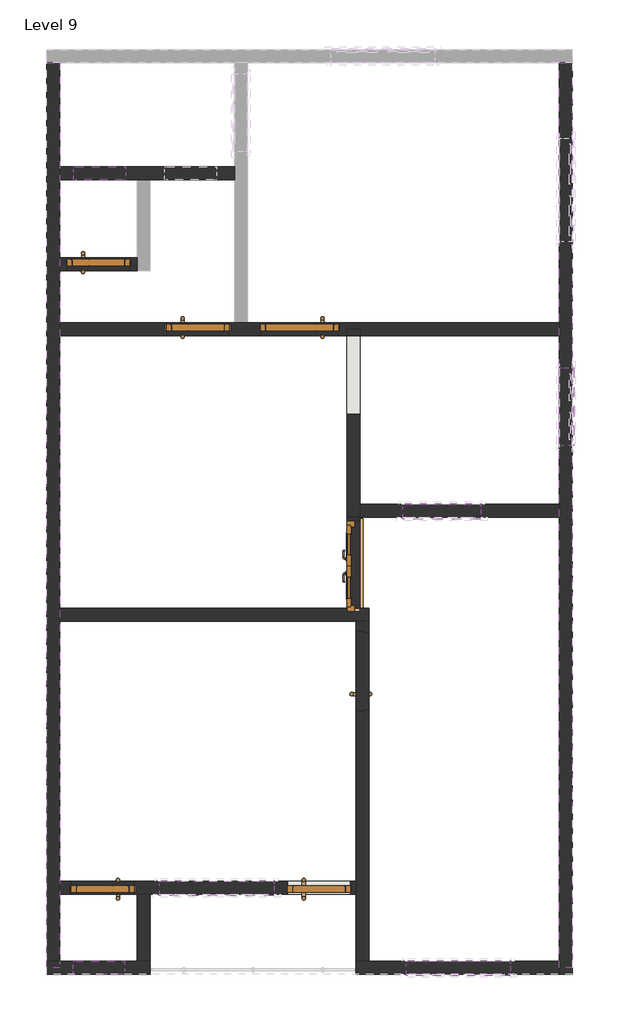
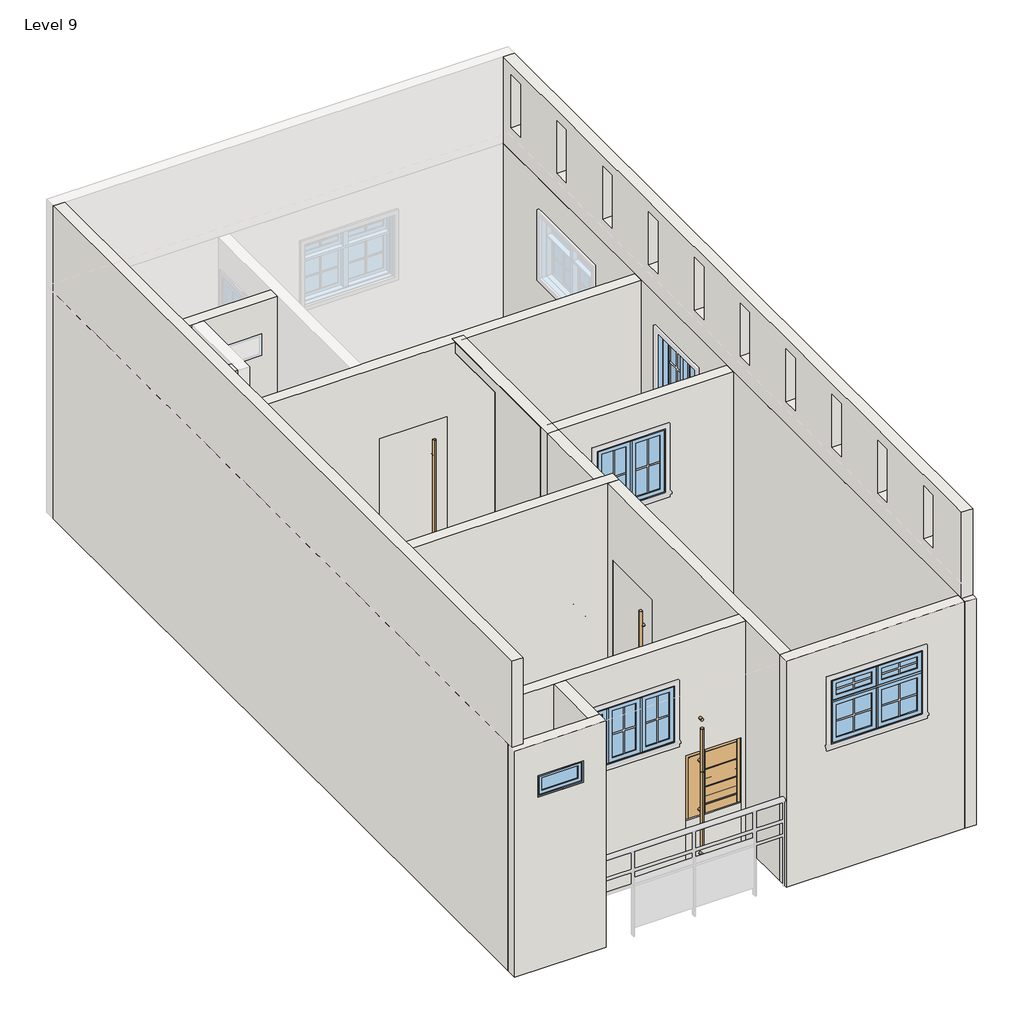
# One storey, part 1 of 2: 25 walls, 8 doors, 8 windows.
"""IFC4 building model written with IfcOpenShell, lengths in millimetres."""

from ifc_helpers import new_model, si_unit, frame, origin, place, context, project, spatial, polyline, outline, extrude, faceted_brep, transform, mapped, element, save
from components import door_9b787682, door_dc81b0c5, door_3_5c4206ef, door_3_79df91aa, door_2576ec39, door_55c03dfd, fixed_2_65c13adb, window_61697a4f, m_window_casement_double_3_e0bd8fa3, m_window_casement_double_awning_double_4_7efa9bbd

model = new_model("IFC4")

# Units and contexts
model_context = context("Model", 3, world=origin())
ifc_project = project(units=[si_unit("LENGTHUNIT", "METRE", prefix="MILLI")], contexts=[model_context])

# Site, building, storey
site = spatial("IfcSite", under=ifc_project)
building = spatial("IfcBuilding", under=site)
storey = spatial("IfcBuildingStorey", under=building, Name="Level 9", Elevation=16611.6)

# Doors
placement = place(None, origin())
door_shape = door_9b787682(model_context)
element("IfcDoor", 1, ObjectType="2'5\"", at=placement, inside=storey, context=model_context, shape_type="MappedRepresentation", body=[
    mapped(door_shape, transform((-22033.2963079, 3049.4742053, 16611.6), x_axis=(1.0, 0.0, 0.0), y_axis=(0.0, 1.0, 0.0), z_axis=(0.0, 0.0, 1.0))),
])
element("IfcDoor", 2, ObjectType="2'5\"", at=placement, inside=storey, context=model_context, shape_type="MappedRepresentation", body=[
    mapped(door_shape, transform((-23201.6963079, 3811.4742053, 16611.6), x_axis=(1.0, 0.0, 0.0), y_axis=(0.0, 1.0, 0.0), z_axis=(0.0, 0.0, 1.0))),
])
element("IfcDoor", 3, ObjectType="2'5\"", at=placement, inside=storey, context=model_context, shape_type="MappedRepresentation", body=[
    mapped(door_shape, transform((-23150.8963079, -3503.7257947, 16611.6), x_axis=(-1.0, 0.0, 0.0), y_axis=(0.0, -1.0, 0.0), z_axis=(0.0, 0.0, 1.0))),
])
door_2_shape = door_dc81b0c5(model_context)
element("IfcDoor", 4, ObjectType="2'5\"", at=placement, inside=storey, context=model_context, shape_type="MappedRepresentation", body=[
    mapped(door_2_shape, transform((-20610.8963079, -3503.7257947, 16657.8445349), x_axis=(1.0, 0.0, 0.0), y_axis=(0.0, 1.0, 0.0), z_axis=(0.0, 0.0, 1.0))),
])
element("IfcDoor", 5, ObjectType="2'5\"", at=placement, inside=storey, context=model_context, shape_type="MappedRepresentation", body=[
    mapped(door_2_shape, transform((-20610.8963079, -3503.7257947, 17267.4445349), x_axis=(1.0, 0.0, 0.0), y_axis=(0.0, 1.0, 0.0), z_axis=(0.0, 0.0, 1.0))),
])
door_3_shape = door_3_5c4206ef(model_context)
element("IfcDoor", 6, ObjectType="3'", at=placement, inside=storey, context=model_context, shape_type="MappedRepresentation", body=[
    mapped(door_3_shape, transform((-20102.8963079, -963.7257947, 16611.6), x_axis=(0.0, 1.0, 0.0), y_axis=(-1.0, 0.0, 0.0), z_axis=(0.0, 0.0, 1.0))),
])
door_3_2_shape = door_3_79df91aa(model_context)
element("IfcDoor", 7, ObjectType="3'", at=placement, inside=storey, context=model_context, shape_type="MappedRepresentation", body=[
    mapped(door_3_2_shape, transform((-20839.4963079, 3049.4742053, 16611.6), x_axis=(-1.0, 0.0, 0.0), y_axis=(0.0, -1.0, 0.0), z_axis=(0.0, 0.0, 1.0))),
])
door_4_shape = door_2576ec39(model_context)
door_5_shape = door_55c03dfd(model_context)
element("IfcDoor", 8, ObjectType="ExtDbl (8) : 3'6\"", at=placement, inside=storey, context=model_context, shape_type="MappedRepresentation", body=[
    mapped(door_4_shape, transform((-20204.4963079, 268.1742053, 16611.6), x_axis=(0.0, -1.0, 0.0), y_axis=(1.0, 0.0, 0.0), z_axis=(0.0, 0.0, 1.0))),
    mapped(door_5_shape, transform((-20204.4963079, 268.1742053, 16611.6), x_axis=(0.0, -1.0, 0.0), y_axis=(1.0, 0.0, 0.0), z_axis=(0.0, 0.0, 1.0))),
])

# Walls
element("IfcWall", 9, ObjectType="Generic - 6\"", at=placement, inside=storey, context=model_context, shape_type="Brep", body=[
    faceted_brep([(-17791.4963079, 6173.6742053, 16611.6), (-17791.4963079, 3125.6742053, 16611.6), (-17791.4963079, 2973.2742053, 16611.6), (-17791.4963079, 992.0742053, 16611.6), (-17791.4963079, 839.6742053, 16611.6), (-17791.4963079, -4367.3257947, 16611.6), (-17791.4963079, -4519.7257947, 16611.6), (-17791.4963079, -4519.7257947, 19812.0), (-17791.4963079, -4367.3257947, 19812.0), (-17791.4963079, 839.6742053, 19812.0), (-17791.4963079, 992.0742053, 19812.0), (-17791.4963079, 2973.2742053, 19812.0), (-17791.4963079, 3125.6742053, 19812.0), (-17791.4963079, 6173.6742053, 19812.0), (-17791.4963079, 4071.8242053, 19340.4), (-17791.4963079, 4071.8242053, 18440.4), (-17791.4963079, 5291.0242053, 18440.4), (-17791.4963079, 5291.0242053, 19340.4), (-17791.4963079, 1682.6367053, 19340.4), (-17791.4963079, 1682.6367053, 18440.4), (-17791.4963079, 2597.0367053, 18440.4), (-17791.4963079, 2597.0367053, 19340.4), (-17639.0963079, 6173.6742053, 16611.6), (-17639.0963079, 6173.6742053, 19812.0), (-17639.0963079, -4519.7257947, 19812.0), (-17639.0963079, -4519.7257947, 16611.6), (-17639.0963079, 4071.8242053, 19340.4), (-17639.0963079, 5291.0242053, 19340.4), (-17639.0963079, 5291.0242053, 18440.4), (-17639.0963079, 4071.8242053, 18440.4), (-17639.0963079, 1682.6367053, 19340.4), (-17639.0963079, 2597.0367053, 19340.4), (-17639.0963079, 2597.0367053, 18440.4), (-17639.0963079, 1682.6367053, 18440.4)], [[[0, 1, 2, 3, 4, 5, 6, 7, 8, 9, 10, 11, 12, 13], [14, 15, 16, 17], [18, 19, 20, 21]], [[22, 23, 24, 25], [26, 27, 28, 29], [30, 31, 32, 33]], [[6, 5, 4, 3, 2, 1, 0, 22, 25]], [[13, 12, 11, 10, 9, 8, 7, 24, 23]], [[0, 13, 23, 22]], [[7, 6, 25, 24]], [[15, 14, 26, 29]], [[16, 15, 29, 28]], [[17, 16, 28, 27]], [[14, 17, 27, 26]], [[19, 18, 30, 33]], [[20, 19, 33, 32]], [[21, 20, 32, 31]], [[18, 21, 31, 30]]]),
])
element("IfcWall", 10, ObjectType="Generic - 6\"", at=placement, inside=storey, context=model_context, shape_type="Brep", body=[
    faceted_brep([(-17791.4963079, -4367.3257947, 16611.6), (-20026.6963079, -4367.3257947, 16611.6), (-20179.0963079, -4367.3257947, 16611.6), (-20179.0963079, -4367.3257947, 19812.0), (-20026.6963079, -4367.3257947, 19812.0), (-17791.4963079, -4367.3257947, 19812.0), (-19585.5697454, -4367.3257947, 19340.4), (-19585.5697454, -4367.3257947, 18440.4), (-18366.3697454, -4367.3257947, 18440.4), (-18366.3697454, -4367.3257947, 19340.4), (-17791.4963079, -4519.7257947, 16611.6), (-17791.4963079, -4519.7257947, 19812.0), (-20179.0963079, -4519.7257947, 19812.0), (-20179.0963079, -4519.7257947, 16611.6), (-19585.5697454, -4519.7257947, 19340.4), (-18366.3697454, -4519.7257947, 19340.4), (-18366.3697454, -4519.7257947, 18440.4), (-19585.5697454, -4519.7257947, 18440.4)], [[[0, 1, 2, 3, 4, 5], [6, 7, 8, 9]], [[10, 11, 12, 13], [14, 15, 16, 17]], [[2, 1, 0, 10, 13]], [[5, 4, 3, 12, 11]], [[0, 5, 11, 10]], [[3, 2, 13, 12]], [[7, 6, 14, 17]], [[8, 7, 17, 16]], [[9, 8, 16, 15]], [[6, 9, 15, 14]]]),
])
element("IfcWall", 11, ObjectType="Generic - 6\"", at=placement, inside=storey, context=model_context, shape_type="Brep", body=[
    faceted_brep([(-23811.2963079, -4519.7257947, 16611.6), (-22592.0963079, -4519.7257947, 16611.6), (-22592.0963079, -4519.7257947, 19812.0), (-23811.2963079, -4519.7257947, 19812.0), (-23500.5431829, -4519.7257947, 19354.8), (-22890.9431829, -4519.7257947, 19354.8), (-22890.9431829, -4519.7257947, 19050.0), (-23500.5431829, -4519.7257947, 19050.0), (-23811.2963079, -4367.3257947, 16611.6), (-23811.2963079, -4367.3257947, 19812.0), (-23658.8963079, -4367.3257947, 19812.0), (-22744.4963079, -4367.3257947, 19812.0), (-22592.0963079, -4367.3257947, 19812.0), (-22592.0963079, -4367.3257947, 16611.6), (-22744.4963079, -4367.3257947, 16611.6), (-23658.8963079, -4367.3257947, 16611.6), (-23500.5431829, -4367.3257947, 19354.8), (-23500.5431829, -4367.3257947, 19050.0), (-22890.9431829, -4367.3257947, 19050.0), (-22890.9431829, -4367.3257947, 19354.8)], [[[0, 1, 2, 3], [4, 5, 6, 7]], [[8, 9, 10, 11, 12, 13, 14, 15], [16, 17, 18, 19]], [[1, 0, 8, 15, 14, 13]], [[3, 2, 12, 11, 10, 9]], [[0, 3, 9, 8]], [[2, 1, 13, 12]], [[17, 16, 4, 7]], [[18, 17, 7, 6]], [[19, 18, 6, 5]], [[16, 19, 5, 4]]]),
])
element("IfcWall", 12, ObjectType="Generic - 6\"", at=placement, inside=storey, context=model_context, shape_type="Brep", body=[
    faceted_brep([(-23658.8963079, -4367.3257947, 16611.6), (-23658.8963079, -3579.9257947, 16611.6), (-23658.8963079, -3427.5257947, 16611.6), (-23658.8963079, -379.5257947, 16611.6), (-23658.8963079, -227.1257947, 16611.6), (-23658.8963079, 2973.2742053, 16611.6), (-23658.8963079, 3125.6742053, 16611.6), (-23658.8963079, 3735.2742053, 16611.6), (-23658.8963079, 3887.6742053, 16611.6), (-23658.8963079, 4802.0742053, 16611.6), (-23658.8963079, 4954.4742053, 16611.6), (-23658.8963079, 6173.6742053, 16611.6), (-23658.8963079, 6173.6742053, 19812.0), (-23658.8963079, 4954.4742053, 19812.0), (-23658.8963079, 4802.0742053, 19812.0), (-23658.8963079, 3887.6742053, 19812.0), (-23658.8963079, 3735.2742053, 19812.0), (-23658.8963079, 3125.6742053, 19812.0), (-23658.8963079, 2973.2742053, 19812.0), (-23658.8963079, -227.1257947, 19812.0), (-23658.8963079, -379.5257947, 19812.0), (-23658.8963079, -3427.5257947, 19812.0), (-23658.8963079, -3579.9257947, 19812.0), (-23658.8963079, -4367.3257947, 19812.0), (-23811.2963079, -4367.3257947, 16611.6), (-23811.2963079, -4367.3257947, 19812.0), (-23811.2963079, 6173.6742053, 19812.0), (-23811.2963079, 6173.6742053, 16611.6)], [[[0, 1, 2, 3, 4, 5, 6, 7, 8, 9, 10, 11, 12, 13, 14, 15, 16, 17, 18, 19, 20, 21, 22, 23]], [[24, 25, 26, 27]], [[11, 10, 9, 8, 7, 6, 5, 4, 3, 2, 1, 0, 24, 27]], [[23, 22, 21, 20, 19, 18, 17, 16, 15, 14, 13, 12, 26, 25]], [[12, 11, 27, 26]], [[0, 23, 25, 24]]]),
])
element("IfcWall", 13, ObjectType="Generic - 6\"", at=placement, inside=storey, context=model_context, shape_type="Brep", body=[
    faceted_brep([(-17791.4963079, 2973.2742053, 19812.0), (-20128.2963079, 2973.2742053, 19812.0), (-20280.6963079, 2973.2742053, 19812.0), (-23658.8963079, 2973.2742053, 19812.0), (-23658.8963079, 2973.2742053, 16611.6), (-22401.5963079, 2973.2742053, 16611.6), (-22401.5963079, 2973.2742053, 18135.6), (-21664.9963079, 2973.2742053, 18135.6), (-21664.9963079, 2973.2742053, 16611.6), (-21296.6963079, 2973.2742053, 16611.6), (-21296.6963079, 2973.2742053, 18801.1), (-20382.2963079, 2973.2742053, 18801.1), (-20382.2963079, 2973.2742053, 16611.6), (-20280.6963079, 2973.2742053, 16611.6), (-20128.2963079, 2973.2742053, 16611.6), (-17791.4963079, 2973.2742053, 16611.6), (-23658.8963079, 3125.6742053, 19812.0), (-21601.4963079, 3125.6742053, 19812.0), (-21449.0963079, 3125.6742053, 19812.0), (-17791.4963079, 3125.6742053, 19812.0), (-17791.4963079, 3125.6742053, 16611.6), (-20382.2963079, 3125.6742053, 16611.6), (-20382.2963079, 3125.6742053, 18801.1), (-21296.6963079, 3125.6742053, 18801.1), (-21296.6963079, 3125.6742053, 16611.6), (-21449.0963079, 3125.6742053, 16611.6), (-21601.4963079, 3125.6742053, 16611.6), (-21664.9963079, 3125.6742053, 16611.6), (-21664.9963079, 3125.6742053, 18135.6), (-22401.5963079, 3125.6742053, 18135.6), (-22401.5963079, 3125.6742053, 16611.6), (-23658.8963079, 3125.6742053, 16611.6), (-22401.5963079, 3105.6742053, 16611.6), (-22416.5963079, 3105.6742053, 16611.6), (-22416.5963079, 3028.6742053, 16611.6), (-22401.5963079, 3028.6742053, 16611.6), (-20382.2963079, 3028.6742053, 16611.6), (-20367.2963079, 3028.6742053, 16611.6), (-20367.2963079, 3105.6742053, 16611.6), (-20382.2963079, 3105.6742053, 16611.6), (-21296.6963079, 3028.6742053, 16611.6), (-21664.9963079, 3028.6742053, 16611.6), (-21649.9963079, 3028.6742053, 16611.6), (-21649.9963079, 3105.6742053, 16611.6), (-21664.9963079, 3105.6742053, 16611.6), (-21296.6963079, 3105.6742053, 16611.6), (-21311.6963079, 3105.6742053, 16611.6), (-21311.6963079, 3028.6742053, 16611.6), (-21296.6963079, 3105.6742053, 18801.1), (-20382.2963079, 3105.6742053, 18801.1), (-20382.2963079, 3028.6742053, 18801.1), (-21296.6963079, 3028.6742053, 18801.1), (-21311.6963079, 3105.6742053, 18816.1), (-20367.2963079, 3105.6742053, 18816.1), (-20367.2963079, 3028.6742053, 18816.1), (-21311.6963079, 3028.6742053, 18816.1), (-21664.9963079, 3105.6742053, 18135.6), (-22401.5963079, 3105.6742053, 18135.6), (-22401.5963079, 3028.6742053, 18135.6), (-21664.9963079, 3028.6742053, 18135.6), (-22416.5963079, 3105.6742053, 18150.6), (-21649.9963079, 3105.6742053, 18150.6), (-21649.9963079, 3028.6742053, 18150.6), (-22416.5963079, 3028.6742053, 18150.6)], [[[0, 1, 2, 3, 4, 5, 6, 7, 8, 9, 10, 11, 12, 13, 14, 15]], [[16, 17, 18, 19, 20, 21, 22, 23, 24, 25, 26, 27, 28, 29, 30, 31]], [[4, 31, 30, 32, 33, 34, 35, 5]], [[20, 15, 14, 13, 12, 36, 37, 38, 39, 21]], [[40, 9, 8, 41, 42, 43, 44, 27, 26, 25, 24, 45, 46, 47]], [[3, 2, 1, 0, 19, 18, 17, 16]], [[0, 15, 20, 19]], [[4, 3, 16, 31]], [[48, 23, 22, 49]], [[50, 11, 10, 51]], [[23, 48, 45, 24]], [[51, 10, 9, 40]], [[49, 22, 21, 39]], [[11, 50, 36, 12]], [[52, 53, 54, 55]], [[52, 55, 47, 46]], [[50, 51, 40, 47, 55, 54, 37, 36]], [[54, 53, 38, 37]], [[48, 49, 39, 38, 53, 52, 46, 45]], [[28, 56, 57, 29]], [[6, 58, 59, 7]], [[56, 28, 27, 44]], [[7, 59, 41, 8]], [[29, 57, 32, 30]], [[58, 6, 5, 35]], [[60, 61, 62, 63]], [[62, 61, 43, 42]], [[59, 58, 35, 34, 63, 62, 42, 41]], [[60, 63, 34, 33]], [[57, 56, 44, 43, 61, 60, 33, 32]]]),
])
element("IfcWall", 14, ObjectType="Generic - 6\"", at=placement, inside=storey, context=model_context, shape_type="Brep", body=[
    faceted_brep([(-20280.6963079, 3049.4742053, 19812.0), (-20280.6963079, 3049.4742053, 16611.6), (-20280.6963079, 839.6742053, 16611.6), (-20280.6963079, 839.6742053, 19812.0), (-20280.6963079, 2974.7724011, 19659.6), (-20280.6963079, 2050.5574639, 19659.6), (-20280.6963079, 2050.5574639, 17221.2), (-20280.6963079, 2974.7724011, 17221.2), (-20128.2963079, 839.6742053, 16611.6), (-20128.2963079, 992.0742053, 16611.6), (-20128.2963079, 3049.4742053, 16611.6), (-20128.2963079, 3049.4742053, 19812.0), (-20128.2963079, 992.0742053, 19812.0), (-20128.2963079, 839.6742053, 19812.0), (-20128.2963079, 2050.5574639, 19659.6), (-20128.2963079, 2974.7724011, 19659.6), (-20128.2963079, 2974.7724011, 17221.2), (-20128.2963079, 2050.5574639, 17221.2)], [[[0, 1, 2, 3], [4, 5, 6, 7]], [[8, 9, 10, 11, 12, 13], [14, 15, 16, 17]], [[2, 1, 10, 9, 8]], [[0, 3, 13, 12, 11]], [[3, 2, 8, 13]], [[4, 15, 14, 5]], [[6, 17, 16, 7]], [[15, 4, 7, 16]], [[5, 14, 17, 6]], [[0, 11, 10, 1]]]),
])
element("IfcWall", 15, ObjectType="Generic - 6\"", at=placement, inside=storey, context=model_context, shape_type="SweptSolid", body=[
    extrude(outline(polyline([(16611.6, -20128.2963079), (16611.6, -17791.4963079), (19812.0, -17791.4963079), (19812.0, -20128.2963079), (16611.6, -20128.2963079)]), holes=[polyline([(19340.4, -19624.1658391), (19340.4, -18709.7658391), (18440.4, -18709.7658391), (18440.4, -19624.1658391), (19340.4, -19624.1658391)])]), frame((0.0, 839.6742053, 0.0), z_axis=(0.0, 1.0, 0.0), x_axis=(0.0, 0.0, 1.0)), (0.0, 0.0, 1.0), 152.4),
])
element("IfcWall", 16, ObjectType="Generic - 6\"", at=placement, inside=storey, context=model_context, shape_type="Brep", body=[
    faceted_brep([(-23658.8963079, -379.5257947, 16611.6), (-20179.0963079, -379.5257947, 16611.6), (-20026.6963079, -379.5257947, 16611.6), (-20026.6963079, -379.5257947, 19812.0), (-20179.0963079, -379.5257947, 19812.0), (-23658.8963079, -379.5257947, 19812.0), (-23658.8963079, -227.1257947, 19812.0), (-20280.6963079, -227.1257947, 19812.0), (-20128.2963079, -227.1257947, 19812.0), (-20026.6963079, -227.1257947, 19812.0), (-20026.6963079, -227.1257947, 16611.6), (-20128.2963079, -227.1257947, 16611.6), (-20128.2963079, -227.1257947, 18721.6), (-20280.6963079, -227.1257947, 18721.6), (-20280.6963079, -227.1257947, 16611.6), (-23658.8963079, -227.1257947, 16611.6), (-20280.6963079, -265.2257947, 16611.6), (-20128.2963079, -265.2257947, 16611.6), (-20280.6963079, -265.2257947, 18721.6), (-20128.2963079, -265.2257947, 18721.6)], [[[0, 1, 2, 3, 4, 5]], [[6, 7, 8, 9, 10, 11, 12, 13, 14, 15]], [[2, 1, 0, 15, 14, 16, 17, 11, 10]], [[5, 4, 3, 9, 8, 7, 6]], [[0, 5, 6, 15]], [[3, 2, 10, 9]], [[18, 16, 14, 13]], [[17, 19, 12, 11]], [[19, 18, 13, 12]], [[16, 18, 19, 17]]]),
])
element("IfcWall", 17, ObjectType="Generic - 6\"", at=placement, inside=storey, context=model_context, shape_type="Brep", body=[
    faceted_brep([(-20179.0963079, -4367.3257947, 19812.0), (-20179.0963079, -3579.9257947, 19812.0), (-20179.0963079, -3427.5257947, 19812.0), (-20179.0963079, -379.5257947, 19812.0), (-20179.0963079, -379.5257947, 16611.6), (-20179.0963079, -506.5257947, 16611.6), (-20179.0963079, -506.5257947, 18801.1), (-20179.0963079, -1420.9257947, 18801.1), (-20179.0963079, -1420.9257947, 16611.6), (-20179.0963079, -3427.5257947, 16611.6), (-20179.0963079, -3579.9257947, 16611.6), (-20179.0963079, -4367.3257947, 16611.6), (-20026.6963079, -379.5257947, 19812.0), (-20026.6963079, -4367.3257947, 19812.0), (-20026.6963079, -4367.3257947, 16611.6), (-20026.6963079, -1420.9257947, 16611.6), (-20026.6963079, -1420.9257947, 18801.1), (-20026.6963079, -506.5257947, 18801.1), (-20026.6963079, -506.5257947, 16611.6), (-20026.6963079, -379.5257947, 16611.6), (-20082.0963079, -506.5257947, 16611.6), (-20082.0963079, -491.5257947, 16611.6), (-20159.0963079, -491.5257947, 16611.6), (-20159.0963079, -506.5257947, 16611.6), (-20159.0963079, -1420.9257947, 16611.6), (-20159.0963079, -1435.9257947, 16611.6), (-20082.0963079, -1435.9257947, 16611.6), (-20082.0963079, -1420.9257947, 16611.6), (-20159.0963079, -506.5257947, 18801.1), (-20159.0963079, -1420.9257947, 18801.1), (-20082.0963079, -1420.9257947, 18801.1), (-20082.0963079, -506.5257947, 18801.1), (-20159.0963079, -1435.9257947, 18816.1), (-20159.0963079, -491.5257947, 18816.1), (-20082.0963079, -491.5257947, 18816.1), (-20082.0963079, -1435.9257947, 18816.1)], [[[0, 1, 2, 3, 4, 5, 6, 7, 8, 9, 10, 11]], [[12, 13, 14, 15, 16, 17, 18, 19]], [[4, 19, 18, 20, 21, 22, 23, 5]], [[14, 11, 10, 9, 8, 24, 25, 26, 27, 15]], [[3, 2, 1, 0, 13, 12]], [[0, 11, 14, 13]], [[4, 3, 12, 19]], [[6, 28, 29, 7]], [[16, 30, 31, 17]], [[28, 6, 5, 23]], [[17, 31, 20, 18]], [[7, 29, 24, 8]], [[30, 16, 15, 27]], [[32, 33, 34, 35]], [[34, 33, 22, 21]], [[31, 30, 27, 26, 35, 34, 21, 20]], [[32, 35, 26, 25]], [[29, 28, 23, 22, 33, 32, 25, 24]]]),
])
element("IfcWall", 18, ObjectType="Generic - 6\"", at=placement, inside=storey, context=model_context, shape_type="Brep", body=[
    faceted_brep([(-20179.0963079, -3579.9257947, 19812.0), (-22592.0963079, -3579.9257947, 19812.0), (-22744.4963079, -3579.9257947, 19812.0), (-23658.8963079, -3579.9257947, 19812.0), (-23658.8963079, -3579.9257947, 16611.6), (-23519.1963079, -3579.9257947, 16611.6), (-23519.1963079, -3579.9257947, 18135.6), (-22782.5963079, -3579.9257947, 18135.6), (-22782.5963079, -3579.9257947, 16611.6), (-22744.4963079, -3579.9257947, 16611.6), (-22592.0963079, -3579.9257947, 16611.6), (-20179.0963079, -3579.9257947, 16611.6), (-22484.1463079, -3579.9257947, 18440.4), (-22484.1463079, -3579.9257947, 19240.4), (-21137.9463079, -3579.9257947, 19240.4), (-21137.9463079, -3579.9257947, 18440.4), (-20979.1963079, -3579.9257947, 18181.8445349), (-20242.5963079, -3579.9257947, 18181.8445349), (-20242.5963079, -3579.9257947, 16657.8445349), (-20979.1963079, -3579.9257947, 16657.8445349), (-23658.8963079, -3427.5257947, 19812.0), (-20179.0963079, -3427.5257947, 19812.0), (-20179.0963079, -3427.5257947, 16611.6), (-22782.5963079, -3427.5257947, 16611.6), (-22782.5963079, -3427.5257947, 18135.6), (-23519.1963079, -3427.5257947, 18135.6), (-23519.1963079, -3427.5257947, 16611.6), (-23658.8963079, -3427.5257947, 16611.6), (-22484.1463079, -3427.5257947, 19240.4), (-22484.1463079, -3427.5257947, 18440.4), (-21137.9463079, -3427.5257947, 18440.4), (-21137.9463079, -3427.5257947, 19240.4), (-20242.5963079, -3427.5257947, 18181.8445349), (-20979.1963079, -3427.5257947, 18181.8445349), (-20979.1963079, -3427.5257947, 16657.8445349), (-20242.5963079, -3427.5257947, 16657.8445349), (-23519.1963079, -3482.9257947, 16611.6), (-23534.1963079, -3482.9257947, 16611.6), (-23534.1963079, -3559.9257947, 16611.6), (-23519.1963079, -3559.9257947, 16611.6), (-22782.5963079, -3559.9257947, 16611.6), (-22767.5963079, -3559.9257947, 16611.6), (-22767.5963079, -3482.9257947, 16611.6), (-22782.5963079, -3482.9257947, 16611.6), (-20979.1963079, -3559.9257947, 18181.8445349), (-20242.5963079, -3559.9257947, 18181.8445349), (-20242.5963079, -3482.9257947, 18181.8445349), (-20979.1963079, -3482.9257947, 18181.8445349), (-20242.5963079, -3559.9257947, 16657.8445349), (-20242.5963079, -3482.9257947, 16657.8445349), (-20227.5963079, -3559.9257947, 16657.8445349), (-20227.5963079, -3482.9257947, 16657.8445349), (-20979.1963079, -3482.9257947, 16657.8445349), (-20994.1963079, -3482.9257947, 16657.8445349), (-20994.1963079, -3559.9257947, 16657.8445349), (-20979.1963079, -3559.9257947, 16657.8445349), (-20994.1963079, -3559.9257947, 18196.8445349), (-20994.1963079, -3482.9257947, 18196.8445349), (-20227.5963079, -3482.9257947, 18196.8445349), (-20227.5963079, -3559.9257947, 18196.8445349), (-23519.1963079, -3559.9257947, 18135.6), (-22782.5963079, -3559.9257947, 18135.6), (-22782.5963079, -3482.9257947, 18135.6), (-23519.1963079, -3482.9257947, 18135.6), (-22767.5963079, -3559.9257947, 18150.6), (-23534.1963079, -3559.9257947, 18150.6), (-23534.1963079, -3482.9257947, 18150.6), (-22767.5963079, -3482.9257947, 18150.6)], [[[0, 1, 2, 3, 4, 5, 6, 7, 8, 9, 10, 11], [12, 13, 14, 15], [16, 17, 18, 19]], [[20, 21, 22, 23, 24, 25, 26, 27], [28, 29, 30, 31], [32, 33, 34, 35]], [[4, 27, 26, 36, 37, 38, 39, 5]], [[22, 11, 10, 9, 8, 40, 41, 42, 43, 23]], [[3, 2, 1, 0, 21, 20]], [[4, 3, 20, 27]], [[0, 11, 22, 21]], [[29, 28, 13, 12]], [[30, 29, 12, 15]], [[31, 30, 15, 14]], [[28, 31, 14, 13]], [[16, 44, 45, 17]], [[32, 46, 47, 33]], [[17, 45, 48, 18]], [[46, 32, 35, 49]], [[18, 48, 50, 51, 49, 35, 34, 52, 53, 54, 55, 19]], [[44, 16, 19, 55]], [[33, 47, 52, 34]], [[56, 57, 58, 59]], [[51, 50, 59, 58]], [[47, 46, 49, 51, 58, 57, 53, 52]], [[54, 53, 57, 56]], [[45, 44, 55, 54, 56, 59, 50, 48]], [[6, 60, 61, 7]], [[24, 62, 63, 25]], [[60, 6, 5, 39]], [[25, 63, 36, 26]], [[7, 61, 40, 8]], [[62, 24, 23, 43]], [[64, 65, 66, 67]], [[66, 65, 38, 37]], [[63, 62, 43, 42, 67, 66, 37, 36]], [[64, 67, 42, 41]], [[61, 60, 39, 38, 65, 64, 41, 40]]]),
])
element("IfcWall", 19, ObjectType="Generic - 6\"", at=placement, inside=storey, context=model_context, shape_type="SweptSolid", body=[
    extrude(outline(polyline([(-22744.4963079, -4367.3257947), (-22744.4963079, -3579.9257947), (-22592.0963079, -3579.9257947), (-22592.0963079, -4367.3257947), (-22744.4963079, -4367.3257947)])), frame((0.0, 0.0, 16611.6), z_axis=(0.0, 0.0, 1.0), x_axis=(1.0, 0.0, 0.0)), (0.0, 0.0, 1.0), 3200.4),
])
element("IfcWall", 20, ObjectType="Generic - 6\"", at=placement, inside=storey, context=model_context, shape_type="Brep", body=[
    faceted_brep([(-23658.8963079, 4802.0742053, 16611.6), (-22744.4963079, 4802.0742053, 16611.6), (-22592.0963079, 4802.0742053, 16611.6), (-21601.4963079, 4802.0742053, 16611.6), (-21601.4963079, 4802.0742053, 19812.0), (-22592.0963079, 4802.0742053, 19812.0), (-22744.4963079, 4802.0742053, 19812.0), (-23658.8963079, 4802.0742053, 19812.0), (-22880.5252141, 4802.0742053, 19354.8), (-22880.5252141, 4802.0742053, 19050.0), (-23490.1252141, 4802.0742053, 19050.0), (-23490.1252141, 4802.0742053, 19354.8), (-21812.6338079, 4802.0742053, 19354.8), (-21812.6338079, 4802.0742053, 19050.0), (-22422.2338079, 4802.0742053, 19050.0), (-22422.2338079, 4802.0742053, 19354.8), (-23658.8963079, 4954.4742053, 16611.6), (-23658.8963079, 4954.4742053, 19812.0), (-21601.4963079, 4954.4742053, 19812.0), (-21601.4963079, 4954.4742053, 16611.6), (-22880.5252141, 4954.4742053, 19354.8), (-23490.1252141, 4954.4742053, 19354.8), (-23490.1252141, 4954.4742053, 19050.0), (-22880.5252141, 4954.4742053, 19050.0), (-21812.6338079, 4954.4742053, 19354.8), (-22422.2338079, 4954.4742053, 19354.8), (-22422.2338079, 4954.4742053, 19050.0), (-21812.6338079, 4954.4742053, 19050.0)], [[[0, 1, 2, 3, 4, 5, 6, 7], [8, 9, 10, 11], [12, 13, 14, 15]], [[16, 17, 18, 19], [20, 21, 22, 23], [24, 25, 26, 27]], [[3, 2, 1, 0, 16, 19]], [[7, 6, 5, 4, 18, 17]], [[0, 7, 17, 16]], [[4, 3, 19, 18]], [[9, 8, 20, 23]], [[10, 9, 23, 22]], [[11, 10, 22, 21]], [[8, 11, 21, 20]], [[13, 12, 24, 27]], [[14, 13, 27, 26]], [[15, 14, 26, 25]], [[12, 15, 25, 24]]]),
])
element("IfcWall", 21, ObjectType="Generic - 6\"", at=placement, inside=storey, context=model_context, shape_type="Brep", body=[
    faceted_brep([(-22744.4963079, 3735.2742053, 19812.0), (-23658.8963079, 3735.2742053, 19812.0), (-23658.8963079, 3735.2742053, 16611.6), (-23569.9963079, 3735.2742053, 16611.6), (-23569.9963079, 3735.2742053, 18135.6), (-22833.3963079, 3735.2742053, 18135.6), (-22833.3963079, 3735.2742053, 16611.6), (-22744.4963079, 3735.2742053, 16611.6), (-23658.8963079, 3887.6742053, 19812.0), (-22744.4963079, 3887.6742053, 19812.0), (-22744.4963079, 3887.6742053, 16611.6), (-22833.3963079, 3887.6742053, 16611.6), (-22833.3963079, 3887.6742053, 18135.6), (-23569.9963079, 3887.6742053, 18135.6), (-23569.9963079, 3887.6742053, 16611.6), (-23658.8963079, 3887.6742053, 16611.6), (-23569.9963079, 3867.6742053, 16611.6), (-23584.9963079, 3867.6742053, 16611.6), (-23584.9963079, 3790.6742053, 16611.6), (-23569.9963079, 3790.6742053, 16611.6), (-22833.3963079, 3790.6742053, 16611.6), (-22818.3963079, 3790.6742053, 16611.6), (-22818.3963079, 3867.6742053, 16611.6), (-22833.3963079, 3867.6742053, 16611.6), (-22833.3963079, 3867.6742053, 18135.6), (-23569.9963079, 3867.6742053, 18135.6), (-23569.9963079, 3790.6742053, 18135.6), (-22833.3963079, 3790.6742053, 18135.6), (-23584.9963079, 3867.6742053, 18150.6), (-22818.3963079, 3867.6742053, 18150.6), (-22818.3963079, 3790.6742053, 18150.6), (-23584.9963079, 3790.6742053, 18150.6)], [[[0, 1, 2, 3, 4, 5, 6, 7]], [[8, 9, 10, 11, 12, 13, 14, 15]], [[2, 15, 14, 16, 17, 18, 19, 3]], [[10, 7, 6, 20, 21, 22, 23, 11]], [[1, 0, 9, 8]], [[0, 7, 10, 9]], [[2, 1, 8, 15]], [[12, 24, 25, 13]], [[4, 26, 27, 5]], [[24, 12, 11, 23]], [[5, 27, 20, 6]], [[13, 25, 16, 14]], [[26, 4, 3, 19]], [[28, 29, 30, 31]], [[30, 29, 22, 21]], [[27, 26, 19, 18, 31, 30, 21, 20]], [[28, 31, 18, 17]], [[25, 24, 23, 22, 29, 28, 17, 16]]]),
])
element("IfcWall", 22, ObjectType="Generic - 6\"", at=placement, inside=storey, context=model_context, shape_type="Brep", body=[
    faceted_brep([(-20280.6963079, -227.1257947, 19812.0), (-20280.6963079, 839.6742053, 19812.0), (-20280.6963079, 839.6742053, 16611.6), (-20280.6963079, 801.5742053, 16611.6), (-20280.6963079, 801.5742053, 18721.6), (-20280.6963079, -227.1257947, 18721.6), (-20128.2963079, 839.6742053, 19812.0), (-20128.2963079, -227.1257947, 19812.0), (-20128.2963079, -227.1257947, 18721.6), (-20128.2963079, 801.5742053, 18721.6), (-20128.2963079, 801.5742053, 16611.6), (-20128.2963079, 839.6742053, 16611.6), (-20179.0963079, -227.1257947, 19812.0), (-20179.0963079, -227.1257947, 18721.6)], [[[0, 1, 2, 3, 4, 5]], [[6, 7, 8, 9, 10, 11]], [[2, 11, 10, 3]], [[1, 0, 12, 7, 6]], [[2, 1, 6, 11]], [[7, 12, 0, 5, 13, 8]], [[4, 9, 8, 13, 5]], [[9, 4, 3, 10]]]),
])
element("IfcWall", 23, ObjectType="Generic - 6\"", at=placement, inside=storey, context=model_context, shape_type="Brep", body=[
    faceted_brep([(-23658.8963079, 2973.2742053, 16611.6), (-20280.6963079, 2973.2742053, 16611.6), (-20128.2963079, 2973.2742053, 16611.6), (-17791.4963079, 2973.2742053, 16611.6), (-17791.4963079, 2973.2742053, 19812.0), (-20128.2963079, 2973.2742053, 19812.0), (-20280.6963079, 2973.2742053, 19812.0), (-23658.8963079, 2973.2742053, 19812.0), (-23658.8963079, 3125.6742053, 16611.6), (-23658.8963079, 3125.6742053, 19812.0), (-21601.4963079, 3125.6742053, 19812.0), (-21449.0963079, 3125.6742053, 19812.0), (-17791.4963079, 3125.6742053, 19812.0), (-17791.4963079, 3125.6742053, 16611.6), (-21449.0963079, 3125.6742053, 16611.6), (-21601.4963079, 3125.6742053, 16611.6)], [[[0, 1, 2, 3, 4, 5, 6, 7]], [[8, 9, 10, 11, 12, 13, 14, 15]], [[3, 2, 1, 0, 8, 15, 14, 13]], [[7, 6, 5, 4, 12, 11, 10, 9]], [[0, 7, 9, 8]], [[4, 3, 13, 12]]]),
])
element("IfcWall", 24, ObjectType="Generic - 6\"", at=placement, inside=storey, context=model_context, shape_type="SweptSolid", body=[
    extrude(outline(polyline([(2973.2742053, 16611.6), (992.0742053, 16611.6), (992.0742053, 19812.0), (2973.2742053, 19812.0), (2973.2742053, 19659.6), (2050.5574639, 19659.6), (2050.5574639, 17221.2), (2973.2742053, 17221.2), (2973.2742053, 16611.6)])), frame((-20280.6963079, 0.0, 0.0), z_axis=(1.0, 0.0, 0.0), x_axis=(0.0, 1.0, 0.0)), (0.0, 0.0, 1.0), 152.4),
])
element("IfcWall", 25, ObjectType="Generic - 6\"", at=placement, inside=storey, context=model_context, shape_type="SweptSolid", body=[
    extrude(outline(polyline([(16611.6, -20128.2963079), (16611.6, -17791.4963079), (19812.0, -17791.4963079), (19812.0, -20128.2963079), (16611.6, -20128.2963079)]), holes=[polyline([(19340.4, -19624.1658391), (19340.4, -18709.7658391), (18440.4, -18709.7658391), (18440.4, -19624.1658391), (19340.4, -19624.1658391)])]), frame((0.0, 839.6742053, 0.0), z_axis=(0.0, 1.0, 0.0), x_axis=(0.0, 0.0, 1.0)), (0.0, 0.0, 1.0), 152.4),
])
element("IfcWall", 26, ObjectType="Generic - 6\"", at=placement, inside=storey, context=model_context, shape_type="Brep", body=[
    faceted_brep([(-23658.8963079, -379.5257947, 16611.6), (-20179.0963079, -379.5257947, 16611.6), (-20179.0963079, -379.5257947, 19812.0), (-23658.8963079, -379.5257947, 19812.0), (-23658.8963079, -227.1257947, 19812.0), (-20280.6963079, -227.1257947, 19812.0), (-20179.0963079, -227.1257947, 19812.0), (-20179.0963079, -227.1257947, 18721.6), (-20280.6963079, -227.1257947, 18721.6), (-20280.6963079, -227.1257947, 16611.6), (-23658.8963079, -227.1257947, 16611.6), (-20280.6963079, -265.2257947, 16611.6), (-20179.0963079, -265.2257947, 16611.6), (-20179.0963079, -265.2257947, 18721.6), (-20280.6963079, -265.2257947, 18721.6)], [[[0, 1, 2, 3]], [[4, 5, 6, 7, 8, 9, 10]], [[1, 0, 10, 9, 11, 12]], [[3, 2, 6, 5, 4]], [[2, 1, 12, 13, 7, 6]], [[14, 11, 9, 8]], [[11, 14, 13, 12]], [[14, 8, 7, 13]], [[0, 3, 4, 10]]]),
])
element("IfcWall", 27, ObjectType="Generic - 6\"", at=placement, inside=storey, context=model_context, shape_type="Brep", body=[
    faceted_brep([(-20179.0963079, -379.5257947, 16611.6), (-20179.0963079, -3427.5257947, 16611.6), (-20179.0963079, -3579.9257947, 16611.6), (-20179.0963079, -4367.3257947, 16611.6), (-20179.0963079, -4367.3257947, 19812.0), (-20179.0963079, -3579.9257947, 19812.0), (-20179.0963079, -3427.5257947, 19812.0), (-20179.0963079, -379.5257947, 19812.0), (-20026.6963079, -379.5257947, 16611.6), (-20026.6963079, -379.5257947, 19812.0), (-20026.6963079, -4367.3257947, 19812.0), (-20026.6963079, -4367.3257947, 16611.6)], [[[0, 1, 2, 3, 4, 5, 6, 7]], [[8, 9, 10, 11]], [[3, 2, 1, 0, 8, 11]], [[7, 6, 5, 4, 10, 9]], [[4, 3, 11, 10]], [[0, 7, 9, 8]]]),
])
element("IfcWall", 28, ObjectType="Generic - 6\"", at=placement, inside=storey, context=model_context, shape_type="Brep", body=[
    faceted_brep([(-23658.8963079, -3579.9257947, 16611.6), (-22744.4963079, -3579.9257947, 16611.6), (-22592.0963079, -3579.9257947, 16611.6), (-20179.0963079, -3579.9257947, 16611.6), (-20179.0963079, -3579.9257947, 19812.0), (-22592.0963079, -3579.9257947, 19812.0), (-22744.4963079, -3579.9257947, 19812.0), (-23658.8963079, -3579.9257947, 19812.0), (-22484.1463079, -3579.9257947, 18440.4), (-22484.1463079, -3579.9257947, 19240.4), (-21137.9463079, -3579.9257947, 19240.4), (-21137.9463079, -3579.9257947, 18440.4), (-20979.1963079, -3579.9257947, 18791.4445349), (-20242.5963079, -3579.9257947, 18791.4445349), (-20242.5963079, -3579.9257947, 17267.4445349), (-20979.1963079, -3579.9257947, 17267.4445349), (-20179.0963079, -3427.5257947, 16611.6), (-23658.8963079, -3427.5257947, 16611.6), (-23658.8963079, -3427.5257947, 19812.0), (-20179.0963079, -3427.5257947, 19812.0), (-22484.1463079, -3427.5257947, 19240.4), (-22484.1463079, -3427.5257947, 18440.4), (-21137.9463079, -3427.5257947, 18440.4), (-21137.9463079, -3427.5257947, 19240.4), (-20242.5963079, -3427.5257947, 18791.4445349), (-20979.1963079, -3427.5257947, 18791.4445349), (-20979.1963079, -3427.5257947, 17267.4445349), (-20242.5963079, -3427.5257947, 17267.4445349), (-20979.1963079, -3559.9257947, 18791.4445349), (-20242.5963079, -3559.9257947, 18791.4445349), (-20242.5963079, -3482.9257947, 18791.4445349), (-20979.1963079, -3482.9257947, 18791.4445349), (-20242.5963079, -3559.9257947, 17267.4445349), (-20242.5963079, -3482.9257947, 17267.4445349), (-20227.5963079, -3559.9257947, 17267.4445349), (-20227.5963079, -3482.9257947, 17267.4445349), (-20979.1963079, -3482.9257947, 17267.4445349), (-20994.1963079, -3482.9257947, 17267.4445349), (-20994.1963079, -3559.9257947, 17267.4445349), (-20979.1963079, -3559.9257947, 17267.4445349), (-20994.1963079, -3559.9257947, 18806.4445349), (-20994.1963079, -3482.9257947, 18806.4445349), (-20227.5963079, -3482.9257947, 18806.4445349), (-20227.5963079, -3559.9257947, 18806.4445349)], [[[0, 1, 2, 3, 4, 5, 6, 7], [8, 9, 10, 11], [12, 13, 14, 15]], [[16, 17, 18, 19], [20, 21, 22, 23], [24, 25, 26, 27]], [[3, 2, 1, 0, 17, 16]], [[7, 6, 5, 4, 19, 18]], [[4, 3, 16, 19]], [[21, 20, 9, 8]], [[22, 21, 8, 11]], [[23, 22, 11, 10]], [[20, 23, 10, 9]], [[12, 28, 29, 13]], [[24, 30, 31, 25]], [[13, 29, 32, 14]], [[30, 24, 27, 33]], [[14, 32, 34, 35, 33, 27, 26, 36, 37, 38, 39, 15]], [[28, 12, 15, 39]], [[25, 31, 36, 26]], [[40, 41, 42, 43]], [[35, 34, 43, 42]], [[31, 30, 33, 35, 42, 41, 37, 36]], [[38, 37, 41, 40]], [[29, 28, 39, 38, 40, 43, 34, 32]], [[0, 7, 18, 17]]]),
])
element("IfcWall", 29, ObjectType="Generic - 6\"", at=placement, inside=storey, context=model_context, shape_type="SweptSolid", body=[
    extrude(outline(polyline([(-22744.4963079, -4367.3257947), (-22744.4963079, -3579.9257947), (-22592.0963079, -3579.9257947), (-22592.0963079, -4367.3257947), (-22744.4963079, -4367.3257947)])), frame((0.0, 0.0, 16611.6), z_axis=(0.0, 0.0, 1.0), x_axis=(1.0, 0.0, 0.0)), (0.0, 0.0, 1.0), 3200.4),
])
element("IfcWall", 30, ObjectType="Generic - 6\"", at=placement, inside=storey, context=model_context, shape_type="SweptSolid", body=[
    extrude(outline(polyline([(-22744.4963079, 3735.2742053), (-23658.8963079, 3735.2742053), (-23658.8963079, 3887.6742053), (-22744.4963079, 3887.6742053), (-22744.4963079, 3735.2742053)])), frame((0.0, 0.0, 16611.6), z_axis=(0.0, 0.0, 1.0), x_axis=(1.0, 0.0, 0.0)), (0.0, 0.0, 1.0), 3200.4),
])
element("IfcWall", 31, ObjectType="Generic - 6\"", at=placement, inside=storey, context=model_context, shape_type="Brep", body=[
    faceted_brep([(-20280.6963079, 839.6742053, 16611.6), (-20280.6963079, -227.1257947, 16611.6), (-20280.6963079, -227.1257947, 19812.0), (-20280.6963079, 839.6742053, 19812.0), (-20128.2963079, 839.6742053, 16611.6), (-20128.2963079, 839.6742053, 19812.0), (-20128.2963079, -227.1257947, 19812.0), (-20128.2963079, -227.1257947, 16611.6), (-20179.0963079, -227.1257947, 19812.0)], [[[0, 1, 2, 3]], [[4, 5, 6, 7]], [[1, 0, 4, 7]], [[3, 2, 8, 6, 5]], [[2, 1, 7, 6, 8]], [[0, 3, 5, 4]]]),
])
element("IfcWall", 32, ObjectType="Generic - 6\"", at=placement, inside=storey, context=model_context, shape_type="SweptSolid", body=[
    extrude(outline(polyline([(6173.6742053, 19812.0), (-4443.5257947, 19812.0), (-4443.5257947, 21031.2), (6173.6742053, 21031.2), (6173.6742053, 19812.0)]), holes=[polyline([(-3566.483991, 20875.4336528), (-3781.9528499, 20875.4336528), (-3781.9528499, 20127.6299662), (-3566.483991, 20127.6299662), (-3566.483991, 20875.4336528)]), polyline([(5774.7247726, 20140.2538824), (5990.1936315, 20140.2538824), (5990.1936315, 20888.0575691), (5774.7247726, 20888.0575691), (5774.7247726, 20140.2538824)]), polyline([(4928.3405623, 20138.8512251), (4928.3405623, 20886.6549117), (4712.8717035, 20886.6549117), (4712.8717035, 20138.8512251), (4928.3405623, 20138.8512251)]), polyline([(3866.4874932, 20137.4485677), (3866.4874932, 20885.2522543), (3651.0186343, 20885.2522543), (3651.0186343, 20137.4485677), (3866.4874932, 20137.4485677)]), polyline([(2804.634424, 20136.0459103), (2804.634424, 20883.849597), (2589.1655651, 20883.849597), (2589.1655651, 20136.0459103), (2804.634424, 20136.0459103)]), polyline([(1742.7813548, 20134.643253), (1742.7813548, 20882.4469396), (1527.312496, 20882.4469396), (1527.312496, 20134.643253), (1742.7813548, 20134.643253)]), polyline([(680.9282857, 20133.2405956), (680.9282857, 20881.0442823), (465.4594268, 20881.0442823), (465.4594268, 20133.2405956), (680.9282857, 20133.2405956)]), polyline([(-380.9247835, 20131.8379382), (-380.9247835, 20879.6416249), (-596.3936424, 20879.6416249), (-596.3936424, 20131.8379382), (-380.9247835, 20131.8379382)]), polyline([(-1442.7778527, 20130.4352809), (-1442.7778527, 20878.2389675), (-1658.2467115, 20878.2389675), (-1658.2467115, 20130.4352809), (-1442.7778527, 20130.4352809)]), polyline([(-2504.6309218, 20876.8363102), (-2720.0997807, 20876.8363102), (-2720.0997807, 20129.0326235), (-2504.6309218, 20129.0326235), (-2504.6309218, 20876.8363102)])]), frame((-17791.4963079, 0.0, 0.0), z_axis=(1.0, 0.0, 0.0), x_axis=(0.0, 1.0, 0.0)), (0.0, 0.0, 1.0), 152.4),
])
element("IfcWall", 33, ObjectType="Generic - 6\"", at=placement, inside=storey, context=model_context, shape_type="Brep", body=[
    faceted_brep([(-23811.2963079, 6173.6742053, 19812.0), (-23811.2963079, -4443.5257947, 19812.0), (-23811.2963079, -4443.5257947, 21031.2), (-23811.2963079, 6173.6742053, 21031.2), (-23658.8963079, 6173.6742053, 19812.0), (-23658.8963079, 6173.6742053, 21031.2), (-23658.8963079, -4443.5257947, 21031.2), (-23658.8963079, -4443.5257947, 19812.0), (-23658.8963079, -4367.3257947, 19812.0)], [[[0, 1, 2, 3]], [[4, 5, 6, 7, 8]], [[1, 0, 4, 8, 7]], [[2, 1, 7, 6]], [[3, 2, 6, 5]], [[0, 3, 5, 4]]]),
])

# Windows
fixed_2_shape = fixed_2_65c13adb(model_context)
element("IfcWindow", 34, ObjectType="Fixed : 2'", at=placement, inside=storey, context=model_context, shape_type="MappedRepresentation", body=[
    mapped(fixed_2_shape, transform((-23233.8431829, -4443.5257947, 18135.6), x_axis=(-1.0, 0.0, 0.0), y_axis=(0.0, -1.0, 0.0), z_axis=(0.0, 0.0, 1.0))),
])
element("IfcWindow", 35, ObjectType="Fixed : 2'", at=placement, inside=storey, context=model_context, shape_type="MappedRepresentation", body=[
    mapped(fixed_2_shape, transform((-23147.2252141, 4878.2742053, 18135.6), x_axis=(1.0, 0.0, 0.0), y_axis=(0.0, 1.0, 0.0), z_axis=(0.0, 0.0, 1.0))),
])
window_shape = window_61697a4f(model_context)
element("IfcWindow", 36, ObjectType="M_Window-Awning-Triple-Horizontal : 4'5\"", at=placement, inside=storey, context=model_context, shape_type="MappedRepresentation", body=[
    mapped(window_shape, transform((-21811.0463079, -3503.7257947, 17540.4), x_axis=(-1.0, 0.0, 0.0), y_axis=(0.0, -1.0, 0.0), z_axis=(0.0, 0.0, 1.0))),
])
element("IfcWindow", 37, ObjectType="M_Window-Awning-Triple-Horizontal : 4'5\"", at=placement, inside=storey, context=model_context, shape_type="MappedRepresentation", body=[
    mapped(window_shape, transform((-21811.0463079, -3503.7257947, 17540.4), x_axis=(-1.0, 0.0, 0.0), y_axis=(0.0, -1.0, 0.0), z_axis=(0.0, 0.0, 1.0))),
])
m_window_casement_double_3_shape = m_window_casement_double_3_e0bd8fa3(model_context)
element("IfcWindow", 38, ObjectType="M_Window-Casement-Double : 3'", at=placement, inside=storey, context=model_context, shape_type="MappedRepresentation", body=[
    mapped(m_window_casement_double_3_shape, transform((-19166.9658391, 915.8742053, 17540.4), x_axis=(-1.0, 0.0, 0.0), y_axis=(0.0, -1.0, 0.0), z_axis=(0.0, 0.0, 1.0))),
])
element("IfcWindow", 39, ObjectType="M_Window-Casement-Double : 3'", at=placement, inside=storey, context=model_context, shape_type="MappedRepresentation", body=[
    mapped(m_window_casement_double_3_shape, transform((-17715.2963079, 2139.8367053, 17540.4), x_axis=(0.0, -1.0, 0.0), y_axis=(1.0, 0.0, 0.0), z_axis=(0.0, 0.0, 1.0))),
])
element("IfcWindow", 40, ObjectType="M_Window-Casement-Double : 3'", at=placement, inside=storey, context=model_context, shape_type="MappedRepresentation", body=[
    mapped(m_window_casement_double_3_shape, transform((-19166.9658391, 915.8742053, 17540.4), x_axis=(-1.0, 0.0, 0.0), y_axis=(0.0, -1.0, 0.0), z_axis=(0.0, 0.0, 1.0))),
])
m_window_casement_double_awning_double_4_shape = m_window_casement_double_awning_double_4_7efa9bbd(model_context)
element("IfcWindow", 41, ObjectType="M_Window-Casement-Double-Awning-Double : 4'", at=placement, inside=storey, context=model_context, shape_type="MappedRepresentation", body=[
    mapped(m_window_casement_double_awning_double_4_shape, transform((-18975.9697454, -4443.5257947, 17540.4), x_axis=(-1.0, 0.0, 0.0), y_axis=(0.0, -1.0, 0.0), z_axis=(0.0, 0.0, 1.0))),
])

save(model, "model.ifc")

# Revit data of these elements
# Type "2'5\""
#   Type Mark = "9"
#   Water resistance = "up to Class E900, EN 12208:2001"
#   Uniclass2015Version = "v1.21"
#   Uniclass2015Reference = "Ss_25_30_20_30"
#   Uniclass2015Description = "Frame and door leaf system"
#   URL = "www.aluprof.com"
#   Type IFC Predefined Type = "USERDEFINED"
#   Right-hand / Left-hand door [instance default] = ""
#   Resistance to wind load = "up to Class C5/B5, EN 12210:2001"
#   Insert type = "ST"
#   Hardware [instance default] = ""
#   Product page = "https://aluprof.com/en/architects/offer/window-and-door-systems/panel-doors#visualisation"
#   Operation = "SinglePanelOutwardOpening"
#   Opening type = "Outward"
#   NBSReference = "25-50-20/125"
#   NBSDescription = "Frame and door leaf system"
#   Important = "The actual acceptable construction dimensions are dependent on the selection of profiles and hardware, glazing type, construction weight and the construction’s operating conditions. These should be determined by a suitably qualified person, and using ALUPROF’s calculation software"
#   IfcExportType = "USERDEFINED"
#   IfcExportAs = "IfcDoorType"
#   Handle type [instance default] = ""
#   Manufacturer = "ALUPROF SA"
#   Export Type to IFC As = "IfcDoorType"
#   Door sill type [instance default] = ""
#   Description = "External single-leaf panel door outward opening"
#   Model = "MB-86 ST Panel Door AD07"
#   Content of the recyclate in the material = "69.2%"
#   COBie.Type.WarrantyDurationParts = ""
#   COBie.Type.Name = ""
#   COBie.Type.Manufacturer = "ALUPROF SA"
#   COBie.Space.Name = ""
#   COBie.Floor.Name = ""
#   COBie.Facility.Name = ""
#   COBie.CreatedOn = ""
#   COBie.Component.WarrantyStartDate = ""
#   COBie.Component.Name = "MB-86 ST Panel Door AD07"
#   Burglar resistance = "RC2"
#   Air permeability = "up to Class 4, EN 12207:2001"
#   Width of the active leaf = 2' - 1.17717"
#   Placement in wall = 0' - 0.7874"
#   Thickness = 0' - 3.0315"
#   Height of the opening sash = 4' - 9.44094"
#   Handle Offset = 3' - 5.33858"
#   Rough Height = 5' - 2.40945"
#   Rough Width = 2' - 6.1811"
#   Height = 5' - 0"
#   Width = 2' - 5"
#   Construction depth = 0' - 3.0315"
#   Clear opening width = 1' - 8.94882"
#   Clear opening height = 4' - 8.47638"
#   Height of the array = 0' - 9.08136"
#   Schedule No. [instance default] = 1
#   Handrail [instance default] = yes
#   IsExternal = yes
#   Handle [instance default] = no
#   Door closer [instance default] = no
#   Function = 1
#   COBie.Type = yes
#   COBie = yes
#   Access control [instance default] = no
#   Panel = element 346771
#   Wall Closure = (empty or 0)
# Type "3'"
#   Type Mark = "10"
#   Water resistance = "up to Class E900, EN 12208:2001"
#   Uniclass2015Version = "v1.21"
#   Uniclass2015Reference = "Ss_25_30_20_30"
#   Uniclass2015Description = "Frame and door leaf system"
#   URL = "www.aluprof.com"
#   Type IFC Predefined Type = "USERDEFINED"
#   Right-hand / Left-hand door [instance default] = ""
#   Resistance to wind load = "up to Class C5/B5, EN 12210:2001"
#   Insert type = "ST"
#   Hardware [instance default] = ""
#   Product page = "https://aluprof.com/en/architects/offer/window-and-door-systems/panel-doors#visualisation"
#   Operation = "SinglePanelOutwardOpening"
#   Opening type = "Outward"
#   NBSReference = "25-50-20/125"
#   NBSDescription = "Frame and door leaf system"
#   Important = "The actual acceptable construction dimensions are dependent on the selection of profiles and hardware, glazing type, construction weight and the construction’s operating conditions. These should be determined by a suitably qualified person, and using ALUPROF’s calculation software"
#   IfcExportType = "USERDEFINED"
#   IfcExportAs = "IfcDoorType"
#   Handle type [instance default] = ""
#   Manufacturer = "ALUPROF SA"
#   Export Type to IFC As = "IfcDoorType"
#   Door sill type [instance default] = ""
#   Description = "External single-leaf panel door outward opening"
#   Model = "MB-86 ST Panel Door AD07"
#   Content of the recyclate in the material = "69.2%"
#   COBie.Type.WarrantyDurationParts = ""
#   COBie.Type.Name = ""
#   COBie.Type.Manufacturer = "ALUPROF SA"
#   COBie.Space.Name = ""
#   COBie.Floor.Name = ""
#   COBie.Facility.Name = ""
#   COBie.CreatedOn = ""
#   COBie.Component.WarrantyStartDate = ""
#   COBie.Component.Name = "MB-86 ST Panel Door AD07"
#   Burglar resistance = "RC2"
#   Air permeability = "up to Class 4, EN 12207:2001"
#   Width of the active leaf = 2' - 8.17717"
#   Placement in wall = 0' - 0.7874"
#   Thickness = 0' - 3.0315"
#   Height of the opening sash = 6' - 11.64173"
#   Handle Offset = 3' - 5.33858"
#   Rough Height = 7' - 4.61024"
#   Rough Width = 3' - 1.1811"
#   Height = 7' - 2.20079"
#   Width = 3' - 0"
#   Construction depth = 0' - 3.0315"
#   Clear opening width = 2' - 3.94882"
#   Clear opening height = 6' - 10.67717"
#   Height of the array = 1' - 1.44816"
#   Schedule No. [instance default] = 1
#   Handrail [instance default] = yes
#   IsExternal = yes
#   Handle [instance default] = no
#   Door closer [instance default] = no
#   Function = 1
#   COBie.Type = yes
#   COBie = yes
#   Access control [instance default] = no
#   Panel = element 346771
#   Wall Closure = (empty or 0)
# Type "ExtDbl (8) : 3'6\""
#   Type Mark = "14"
#   Operation = "DoubleDoorSingleSwing"
#   Keynote = "L20"
#   Wrap Layers (Int) from Ext = 0' - 6.98819"
#   Wrap Layers (Ext) from Ext = 0' - 4.03543"
#   Top of Lock Rail = 2' - 11.43307"
#   Thickness = 0' - 1.73228"
#   Stile Shutting = 0' - 4.92126"
#   Stile - Top Rail = 0' - 5.90551"
#   Stile - Lock Rail = 0' - 5.90551"
#   Stile - Hanging = 0' - 3.93701"
#   Stile - Bottom Rail = 0' - 11.81102"
#   Rough Width = 3' - 6"
#   Rough Height = 6' - 11.07087"
#   O/A Frame Width = 0' - 2.51969"
#   Handle Z Distance = 3' - 1.40157"
#   Glazing Thickness = 0' - 0.94488"
#   FrameWidth = 0' - 1.65354"
#   FrameOffset - External = 0' - 2.55906"
#   FrameDepth = 0' - 3.50394"
#   Door Panel Width = 1' - 6.91339"
#   Door Panel Thickness = 0' - 1.73228"
#   Door Panel Height = 6' - 6.74016"
#   Cill Thickness = 0' - 2.14567"
#   Cill Projection = 0' - 1.1811"
#   Handle X Distance = 0' - 2.95276"
#   Height = 6' - 11.07087"
#   Structural Tolerance = 0' - 0.25591"
#   Tolerance = 0' - 0.11811"
#   Undercut = 0' - 0.15748"
#   Width = 3' - 6"
#   Cill Extension = 0' - 0.98425"
#   Cavity Closer Width = 0' - 1.9685"
#   Cavity Closer Offset from Ext = 0' - 4.03543"
#   Cavity Closer Depth = 0' - 3.34646"
#   Vis - Ironmongery = yes
#   Vis - Cavity Closers = yes
#   Function = 1
#   Material Glass = Door - Glazing
#   Handle Style = element 349788
#   Material Door = Door - Panel
#   Material Ironmongery = Door - Handle
#   Wall Closure = (empty or 0)
# Type "Generic - 6\""
#   Assembly Code = "B2010"
#   Layers, outside or top first: 0' - 6" no material (function 1)
# Type "Fixed : 2'"
#   Type Mark = "16"
#   Assembly Code = "B2020100"
#   Height = 1' - 0"
#   Default Sill Height = 3' - 0"
#   Width = 2' - 0"
#   Window Inset = 0' - 0 3/4"
#   Glass Pane Material = Glass
#   Sash Material = Sash
#   Wall Closure = (empty or 0)
# Type "M_Window-Awning-Triple-Horizontal : 4'5\""
#   Type Mark = "15"
#   Fire Rating = "0.5h"
#   Assembly Code = "B2020100"
#   Analytic Construction = "Double glazing - domestic"
#   Window Inset [instance default] = 0' - 0"
#   Wall Thickness [instance default] = 0' - 5.90551"
#   Muntin Width = 1' - 0.33333"
#   Visual Light Transmittance = 0.81
#   Thermal Resistance (R) = 1.8146 (h·ft²·°F)/BTU
#   Solar Heat Gain Coefficient = 0.76
#   One Third Width = 1' - 5.66667"
#   Sash Width = 1' - 4.83333"
#   Rough Width = 4' - 5.59055"
#   Rough Height = 2' - 8.08661"
#   Interior Wall Closure [instance default] = 0' - 2.15551"
#   Height = 2' - 7.49606"
#   Heat Transfer Coefficient (U) = 0.5511 BTU/(h·ft²·°F)
#   Muntin Height = 2' - 1.99606"
#   Frame Extension [instance default] = 0' - 0 1/4"
#   Exterior Wall Closure [instance default] = 0' - 1 1/4"
#   Extension Jamb [instance default] = 0' - 2.15551"
#   Default Sill Height = 2' - 11.43307"
#   Width = 4' - 5"
#   Middle Muntin Visibility = yes
#   Side Muntin Visibility = yes
#   Interior Trim Visibility [instance default] = yes
#   Exterior Trim Visibility [instance default] = yes
#   Extension Jamb Visibility [instance default] = yes
#   Muntin Pattern = M_Muntin Pattern_2x2 : M_Muntin Pattern_2x2
#   Interior Trim Material = Wood - Stained
#   Interior Trim = M_Trim-Window-Interior-Flat : Picture Frame
#   Interior Frame Material = Wood - Stained
#   Glass Panel Material = Glass
#   Exterior Trim Material = Clad - White
#   Exterior Trim = M_Trim-Window-Exterior-Flat : with Sill
#   Exterior Frame Material = Clad - White
#   Wall Closure = (empty or 0)
# Type "M_Window-Casement-Double : 3'"
#   Type Mark = "13"
#   Fire Rating = "0.5h"
#   Assembly Code = "B2020100"
#   Analytic Construction = "Double glazing - domestic"
#   Frame Extension [instance default] = 0' - 0 1/4"
#   Window Inset [instance default] = 0' - 0"
#   Wall Thickness [instance default] = 0' - 5.90551"
#   Interior Wall Closure [instance default] = 0' - 2.15551"
#   Half Width = 1' - 6"
#   Visual Light Transmittance = 0.81
#   Thermal Resistance (R) = 1.8146 (h·ft²·°F)/BTU
#   Solar Heat Gain Coefficient = 0.76
#   Rough Width = 3' - 0.59055"
#   Rough Height = 3' - 0.02362"
#   Height = 2' - 11.43307"
#   Heat Transfer Coefficient (U) = 0.5511 BTU/(h·ft²·°F)
#   Exterior Wall Closure [instance default] = 0' - 1.25197"
#   Extension Jamb [instance default] = 0' - 2.15551"
#   Default Sill Height = 2' - 11.43307"
#   Width = 3' - 0"
#   Muntin Visibility = yes
#   Interior Trim Visibility [instance default] = yes
#   Exterior Trim Visibility [instance default] = yes
#   Extension Jamb Visibility [instance default] = yes
#   Interior Trim Material = Wood - Stained
#   Muntin Pattern = M_Muntin Pattern_2x2 : M_Muntin Pattern_2x2
#   Interior Trim = M_Trim-Window-Interior-Flat : Picture Frame
#   Interior Frame Material = Wood - Stained
#   Glass Panel Material = Glass
#   Exterior Trim Material = Clad - White
#   Exterior Trim = M_Trim-Window-Exterior-Flat : with Sill
#   Exterior Frame Material = Clad - White
#   Wall Closure = (empty or 0)
# Type "M_Window-Casement-Double-Awning-Double : 4'"
#   Type Mark = "11"
#   Fire Rating = "0.5h"
#   Assembly Code = "B2020100"
#   Analytic Construction = "Double glazing - domestic"
#   Window Inset [instance default] = 0' - 0"
#   Wall Thickness [instance default] = 0' - 5.90551"
#   Interior Wall Closure [instance default] = 0' - 2.15551"
#   Half Width = 2' - 0"
#   Visual Light Transmittance = 0.81
#   Transom Height = 0' - 11.81102"
#   Thermal Resistance (R) = 1.8146 (h·ft²·°F)/BTU
#   Solar Heat Gain Coefficient = 0.76
#   Rough Width = 4' - 0.59055"
#   Rough Height = 3' - 0.02362"
#   Open Window Height = 1' - 11.62205"
#   Frame Extension [instance default] = 0' - 0 1/4"
#   Height = 2' - 11.43307"
#   Heat Transfer Coefficient (U) = 0.5511 BTU/(h·ft²·°F)
#   Exterior Wall Closure [instance default] = 0' - 1.25197"
#   Extension Jamb [instance default] = 0' - 2.15551"
#   Default Sill Height = 2' - 11.43307"
#   Width = 4' - 0"
#   Top Muntin Visibility = yes
#   Bottom Muntin Visibility = yes
#   Interior Trim Visibility [instance default] = yes
#   Exterior Trim Visibility [instance default] = yes
#   Extension Jamb Visibility [instance default] = yes
#   Interior Trim Material = Wood - Stained
#   Muntin Pattern = M_Muntin Pattern_2x2 : M_Muntin Pattern_2x2
#   Interior Trim = M_Trim-Window-Interior-Flat : Picture Frame
#   Interior Frame Material = Wood - Stained
#   Glass Panel Material = Glass
#   Exterior Trim Material = Clad - White
#   Exterior Trim = M_Trim-Window-Exterior-Flat : with Sill
#   Exterior Frame Material = Clad - White
#   Wall Closure = (empty or 0)
# Elements 1, 2, 3, 4, 5 (IfcDoor, "2'5\"")
#   Right-hand / Left-hand door = ""
#   Hardware = ""
#   Handle type = ""
#   Door sill type = ""
#   Schedule No. = 1
#   Handrail = yes
#   Handle = no
#   Door closer = no
#   Access control = no
#   Phase Created = New Construction
# Elements 6, 7 (IfcDoor, "3'")
#   Right-hand / Left-hand door = ""
#   Hardware = ""
#   Handle type = ""
#   Door sill type = ""
#   Schedule No. = 1
#   Handrail = yes
#   Handle = no
#   Door closer = no
#   Access control = no
